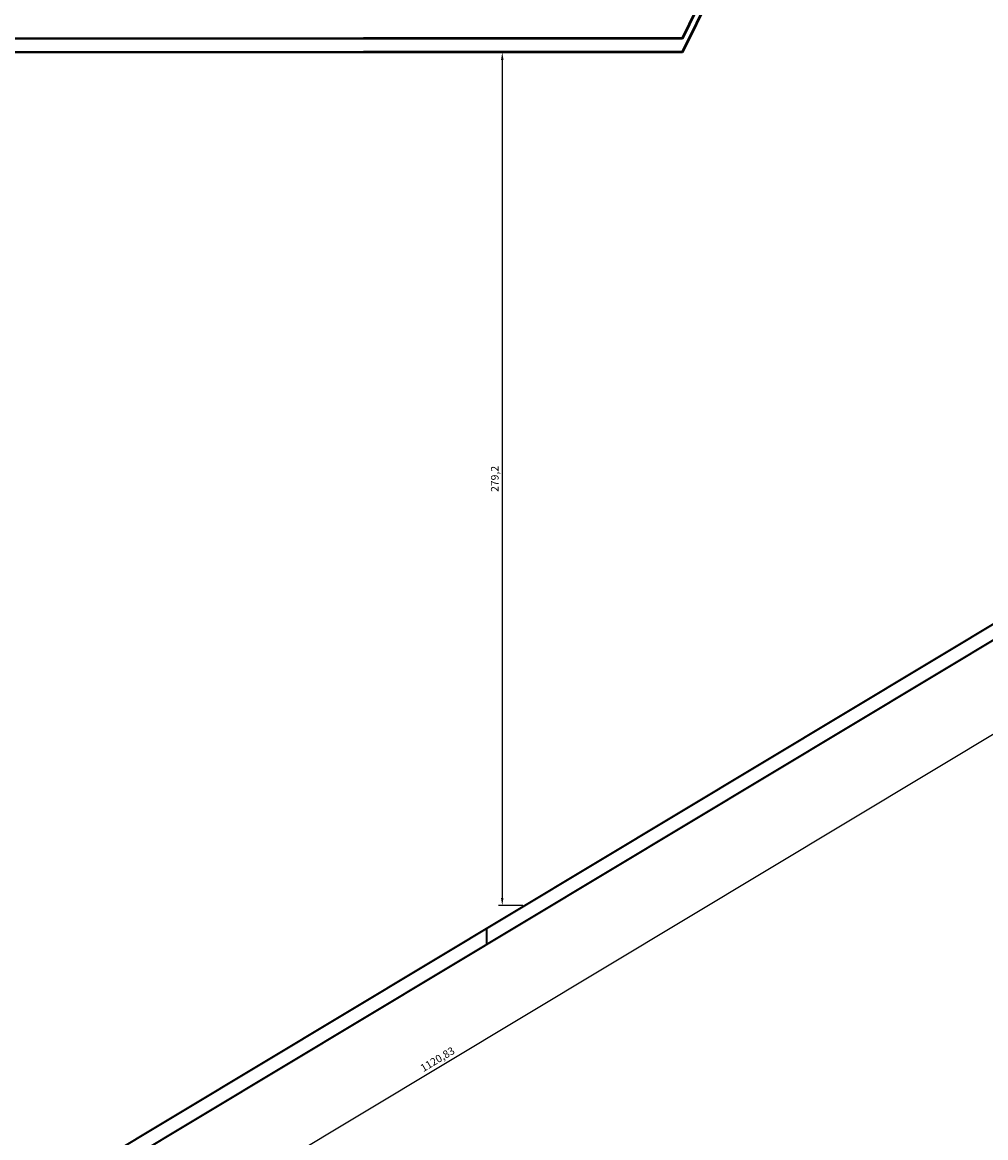
# Model space of a CAD drawing. Units: millimetres. Extents: x 2134 to 3363, y 1052 to 3233.
# Tile 3 of 11: x 2539 to 2854, y 1417 to 1782. Entities that reach past the tile are written whole.
import ezdxf

# ---------------------------------------------------------------- set-up
doc = ezdxf.new("R2010")
doc.units = ezdxf.units.MM
for name, color, linetype, lineweight in [('A-ANNO-DIMS', 2, 'Continuous', 18), ('A-WALL', 7, 'Continuous', 50), ('C-PROP', 6, 'Continuous', 35)]:
    doc.layers.add(name, color=color, linetype=linetype, lineweight=lineweight)
doc.styles.get("Standard").update_dxf_attribs({"font": 'arial.ttf'})
doc.dimstyles.new('ISO-25', dxfattribs={"dimtxt": 2.5, "dimasz": 2.5, "dimexe": 1.25, "dimexo": 0.625, "dimtad": 1, "dimtxsty": 'Standard', "dimcen": 2.5, "dimadec": 0, "dimazin": 0, "dimtfac": 1, "dimtmove": 0, "dimatfit": 3, "dimfxl": 1, "dimarcsym": 0})

# ---------------------------------------------------------------- blocks, each defined once
blk = doc.blocks.new('*D10')
at = {"layer": 'A-ANNO-DIMS', "color": 0, "lineweight": -2, "transparency": 16777216}
for p, q in [((3164.66, 1769.83), (3180.9, 1742.8)), ((3178.12, 1742.58), (2221.66, 1167.89)), ((2203.92, 1192.56), (2220.16, 1165.53))]:
    blk.add_line(p, q, dxfattribs=at)
at = {"layer": 'A-ANNO-DIMS', "color": 0, "transparency": 16777216}
for points in [[(3177.9, 1742.94), (3178.33, 1742.23), (3180.26, 1743.87)], [(2221.44, 1168.24), (2221.87, 1167.53), (2219.52, 1166.6)]]:
    blk.add_solid(points, dxfattribs=at)
at = {"layer": 'Defpoints', "color": 0, "transparency": 16777216}
for p in [(3164.34, 1770.37), (2203.6, 1193.09), (2219.52, 1166.6)]:
    blk.add_point(p, dxfattribs=at)
at = {"layer": 'A-ANNO-DIMS', "color": 0, "transparency": 16777216, "insert": (2674.71, 1442.59), "char_height": 2.5, "attachment_point": 5, "rotation": 31}
blk.add_mtext('1120,83', dxfattribs=at)
blk = doc.blocks.new('*D22')
at = {"layer": 'A-ANNO-DIMS', "color": 0, "lineweight": -2, "transparency": 16777216}
for p, q in [((2701.89, 1772.4), (2694.49, 1772.4)), ((2695.74, 1769.9), (2695.74, 1495.69)), ((2702.42, 1493.19), (2694.49, 1493.19))]:
    blk.add_line(p, q, dxfattribs=at)
at = {"layer": 'A-ANNO-DIMS', "color": 0, "transparency": 16777216}
for points in [[(2695.32, 1769.9), (2696.15, 1769.9), (2695.74, 1772.4)], [(2695.32, 1495.69), (2696.15, 1495.69), (2695.74, 1493.19)]]:
    blk.add_solid(points, dxfattribs=at)
at = {"layer": 'Defpoints', "color": 0, "transparency": 16777216}
for p in [(2702.52, 1772.4), (2695.74, 1493.19), (2703.04, 1493.19)]:
    blk.add_point(p, dxfattribs=at)
at = {"layer": 'A-ANNO-DIMS', "color": 0, "transparency": 16777216, "insert": (2693.61, 1632.79), "char_height": 2.5, "attachment_point": 5, "rotation": 90}
blk.add_mtext('279,2', dxfattribs=at)

msp = doc.modelspace()

# ---------------------------------------------------------------- linework, layer by layer
at = {"layer": 'A-WALL'}
for p, q in [((2754.719, 1776.895), (2830.205, 1931.774)), ((2754.719, 1772.395), (2832.735, 1931.774))]:
    msp.add_line(p, q, dxfattribs=at)
for points in [[(2754.719, 1776.895), (2650.315, 1776.895), (2396.963, 1776.846)], [(2754.719, 1772.395), (2650.315, 1772.395), (2396.964, 1772.346)]]:
    msp.add_lwpolyline(points, dxfattribs=at)
at = {"layer": 'C-PROP'}
for p, q in [((3164.339, 1770.366), (2203.596, 1193.093)), ((3168.839, 1767.82), (2197.066, 1183.92)), ((2690.725, 1480.54), (2690.725, 1485.79))]:
    msp.add_line(p, q, dxfattribs=at)

# ---------------------------------------------------------------- dimensions: what is measured, and where the dimension line sits
at = {"layer": 'A-ANNO-DIMS'}
dim = msp.add_linear_dim(base=(2219.5153, 1166.599), p1=(3164.339, 1770.3661), p2=(2203.5959, 1193.0934), angle=211, dimstyle='ISO-25', override={"dimclrd": 0, "dimclre": 0, "dimclrt": 0}, dxfattribs=at)
dim.commit()
dim.dimension.update_dxf_attribs({"geometry": '*D10', "text_midpoint": (2675.8085, 1440.7677), "dimtype": 161})
dim = msp.add_linear_dim(base=(2695.735, 1493.191), p1=(2702.517, 1772.395), p2=(2703.042, 1493.191), angle=90, dimstyle='ISO-25', override={"dimclrd": 0, "dimclre": 0, "dimclrt": 0}, dxfattribs=at)
dim.commit()
dim.dimension.update_dxf_attribs({"geometry": '*D22', "text_midpoint": (2693.608, 1632.793)})

doc.saveas('drawing.dxf')
